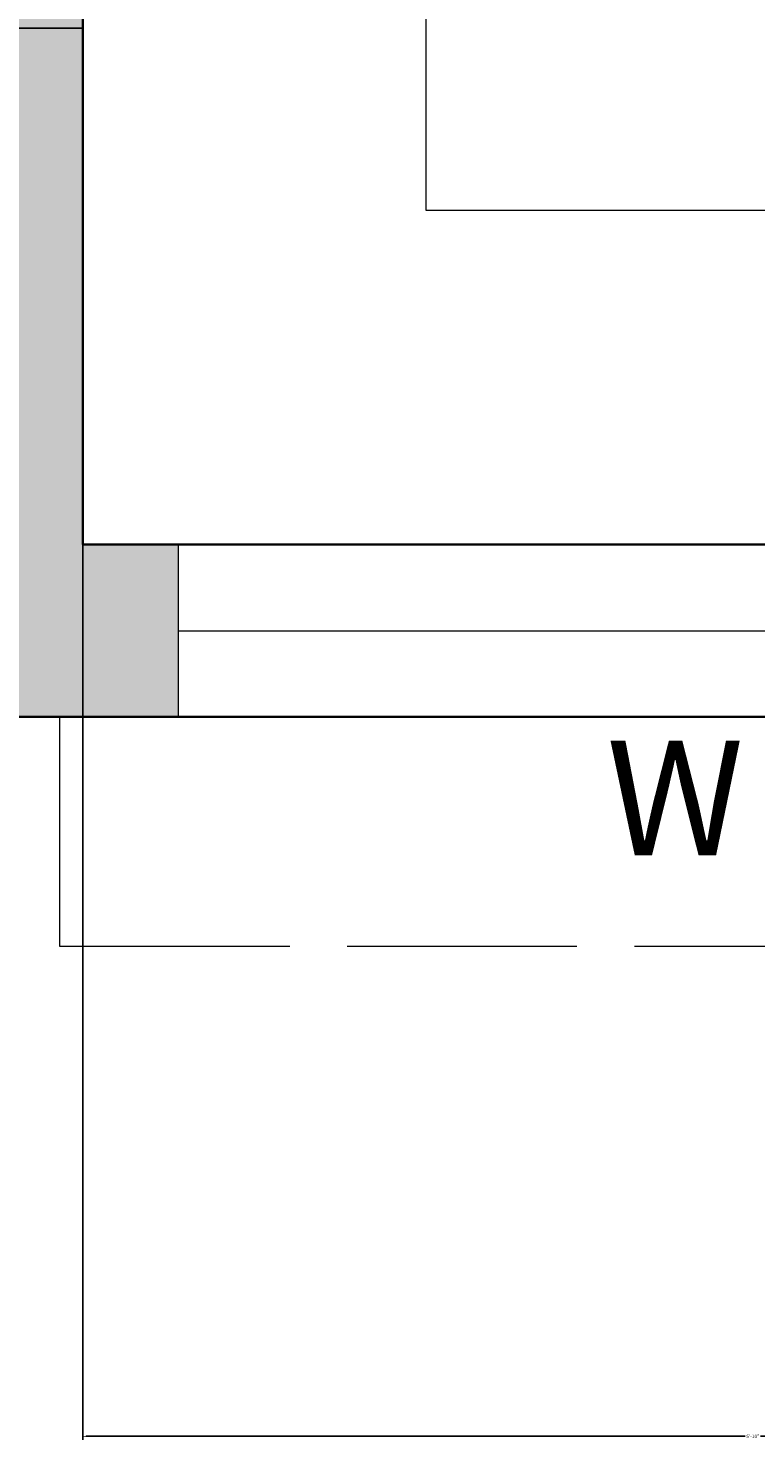
# Model space of a CAD drawing. Units: inches. Extents: x -5 to 482, y -460 to 66.
# Tile 10 of 31: x 142 to 180, y -460 to -386. Entities that reach past the tile are written whole.
import ezdxf

# ---------------------------------------------------------------- set-up
doc = ezdxf.new("R2010")
doc.units = ezdxf.units.IN
doc.header["$MEASUREMENT"] = 0
doc.linetypes.add('ACAD_ISO02W100', pattern=[15, 12, -3])
for name, color, linetype, lineweight in [('A-ANNO-DIMS', 2, 'Continuous', 18), ('A-ANNO-SYMB', 7, 'Continuous', 18), ('A-ANNO-TEXT', 7, 'Continuous', 18), ('A-GLAZ', 4, 'Continuous', 18), ('A-GLAZ-OVHD', 4, 'ACAD_ISO02W100', 13), ('A-WALL', 7, 'Continuous', 35), ('A-WALL-PATT', 152, 'Continuous', 13)]:
    doc.layers.add(name, color=color, linetype=linetype, lineweight=lineweight)
doc.styles.get("Standard").update_dxf_attribs({"font": 'arial.ttf'})
doc.dimstyles.get("Standard").update_dxf_attribs({"dimtxt": 0.18, "dimasz": 0.18, "dimexe": 0.18, "dimexo": 0.0625, "dimgap": 0.09, "dimtad": 0, "dimtih": 1, "dimtoh": 1, "dimdec": 0, "dimzin": 0, "dimdsep": 46, "dimlunit": 3, "dimtxsty": 'Standard', "dimcen": 0.09, "dimadec": 0, "dimazin": 0, "dimtfac": 1, "dimtdec": 0, "dimtofl": 0, "dimtmove": 0, "dimatfit": 3, "dimfxl": 1, "dimtolj": 1, "dimtzin": 0, "dimarcsym": 0})

# ---------------------------------------------------------------- blocks, each defined once
blk = doc.blocks.new('WIN-GLAZ-60IN')
for p, q in [((0, 9), (60, 9)), ((0, 4.5), (60, 4.5)), ((60, 0), (0, 0))]:
    blk.add_line(p, q)
blk = doc.blocks.new('WIN-SHADE-72IN')
for p, q in [((0, 12), (72, 12)), ((0, 12), (0, 0)), ((72, 12), (72, 0))]:
    blk.add_line(p, q)
blk = doc.blocks.new('*D71')
at = {"layer": 'A-ANNO-DIMS', "color": 0, "lineweight": -2, "transparency": 16777216}
for p, q in [((144.377, -385.924), (144.377, -459.629)), ((214.377, -385.924), (214.377, -459.629)), ((144.557, -459.449), (178.978, -459.449)), ((214.197, -459.449), (179.776, -459.449))]:
    blk.add_line(p, q, dxfattribs=at)
at = {"layer": 'A-ANNO-DIMS', "color": 0, "transparency": 16777216}
for points in [[(144.557, -459.419), (144.557, -459.479), (144.377, -459.449)], [(214.197, -459.419), (214.197, -459.479), (214.377, -459.449)]]:
    blk.add_solid(points, dxfattribs=at)
at = {"layer": 'Defpoints', "color": 0, "transparency": 16777216}
for p in [(144.377, -385.861), (214.377, -385.861), (214.377, -459.449)]:
    blk.add_point(p, dxfattribs=at)
at = {"layer": 'A-ANNO-DIMS', "color": 0, "transparency": 16777216, "insert": (179.377, -459.449), "char_height": 0.18, "attachment_point": 5}
blk.add_mtext('\\A1;5\'-10"', dxfattribs=at)
blk = doc.blocks.new('*D72')
at = {"layer": 'A-ANNO-DIMS', "color": 0, "lineweight": -2, "transparency": 16777216}
for p, q in [((144.314, -375.861), (-4.903, -375.861)), ((-4.723, -376.041), (-4.723, -380.679)), ((-4.723, -385.681), (-4.723, -381.043)), ((144.314, -385.861), (-4.903, -385.861))]:
    blk.add_line(p, q, dxfattribs=at)
at = {"layer": 'A-ANNO-DIMS', "color": 0, "transparency": 16777216}
for points in [[(-4.753, -376.041), (-4.693, -376.041), (-4.723, -375.861)], [(-4.753, -385.681), (-4.693, -385.681), (-4.723, -385.861)]]:
    blk.add_solid(points, dxfattribs=at)
at = {"layer": 'Defpoints', "color": 0, "transparency": 16777216}
for p in [(144.377, -375.861), (-4.723, -385.861), (144.377, -385.861)]:
    blk.add_point(p, dxfattribs=at)
at = {"layer": 'A-ANNO-DIMS', "color": 0, "transparency": 16777216, "insert": (-4.723, -380.861), "char_height": 0.18, "attachment_point": 5}
blk.add_mtext('\\A1;0\'-10"', dxfattribs=at)

msp = doc.modelspace()

# ---------------------------------------------------------------- hatches: boundary and pattern name
at = {"layer": 'A-WALL-PATT'}
h = msp.add_hatch(color=256, dxfattribs=at)
h.dxf.hatch_style = 1
h.paths.add_polyline_path([(149.377, -412.849), (144.377, -412.849), (144.377, -283.849), (144.377, -279.349), (133.877, -279.349), (133.877, -283.849), (139.877, -283.849), (139.877, -412.849), (133.51, -412.849), (133.51, -413.916), (102.652, -413.916), (102.652, -421.02), (133.51, -421.02), (133.51, -421.849), (149.377, -421.849)])
h.paths.add_polyline_path([(226.054, -412.849), (218.877, -412.849), (218.877, -350.849), (262.877, -350.849), (262.877, -386.849), (267.377, -386.849), (267.377, -283.849), (270.377, -283.849), (270.377, -279.349), (244.877, -279.349), (244.877, -283.849), (262.877, -283.849), (262.877, -346.349), (218.877, -346.349), (218.877, -283.849), (220.877, -283.849), (220.877, -279.349), (214.377, -279.349), (214.377, -283.849), (214.377, -412.849), (209.377, -412.849), (209.377, -421.849), (226.054, -421.849)])
h.paths.add_polyline_path([(315.815, -412.849), (250.054, -412.849), (250.054, -421.849), (315.815, -421.849)])
h.paths.add_polyline_path([(430.377, -378.349), (421.377, -378.349), (421.377, -412.849), (375.815, -412.849), (375.815, -421.849), (430.377, -421.849)])
h.paths.add_polyline_path([(78.691, -413.916), (47.68, -413.916), (47.68, -412.849), (41.877, -412.849), (41.877, -283.849), (109.877, -283.849), (109.877, -279.349), (41.877, -279.349), (41.877, -241.849), (32.877, -241.849), (32.877, -421.849), (47.68, -421.849), (47.68, -421.02), (78.691, -421.02)])
h.paths.add_polyline_path([(41.877, -144.349), (154.377, -144.349), (154.377, -137.849), (149.877, -137.849), (149.877, -139.849), (41.877, -139.849), (41.877, -97.849), (32.877, -97.849), (32.877, -181.849), (41.877, -181.849)])
h.paths.add_polyline_path([(430.377, -241.849), (421.377, -241.849), (421.377, -279.349), (309.377, -279.349), (309.377, -170.349), (304.877, -170.349), (304.877, -279.349), (294.377, -279.349), (294.377, -283.849), (421.377, -283.849), (421.377, -318.349), (430.377, -318.349)])
h.paths.add_polyline_path([(430.377, -119.849), (421.377, -119.849), (421.377, -139.849), (419.377, -139.849), (419.377, -144.349), (421.377, -144.349), (421.377, -181.849), (430.377, -181.849)])
h.paths.add_polyline_path([(395.377, -139.849), (377.377, -139.849), (377.377, -75.849), (421.377, -75.849), (421.377, -95.849), (430.377, -95.849), (430.377, -45.599), (421.377, -45.599), (421.377, -71.349), (377.377, -71.349), (377.377, -22.849), (372.877, -22.849), (372.877, -139.849), (242.877, -139.849), (242.877, -137.849), (238.377, -137.849), (238.377, -144.349), (304.877, -144.349), (304.877, -146.349), (309.377, -146.349), (309.377, -144.349), (395.377, -144.349)])
h.paths.add_polyline_path([(65.877, 13.151), (32.877, 13.151), (32.877, -37.849), (41.877, -37.849), (41.877, 4.151), (65.877, 4.151)])
h.paths.add_polyline_path([(166.377, 13.151), (125.877, 13.151), (125.877, 4.151), (149.877, 4.151), (149.877, -113.849), (154.377, -113.849), (154.377, 4.151), (166.377, 4.151)])
h.paths.add_polyline_path([(277.877, 13.151), (226.377, 13.151), (226.377, 4.151), (238.377, 4.151), (238.377, -113.849), (242.877, -113.849), (242.877, 4.151), (277.877, 4.151)])
h.paths.add_polyline_path([(430.377, 13.151), (337.877, 13.151), (337.877, 4.151), (372.877, 4.151), (372.877, 1.151), (377.377, 1.151), (377.377, 4.151), (421.377, 4.151), (421.377, -21.599), (430.377, -21.599)])

# ---------------------------------------------------------------- linework, layer by layer
at = {"layer": 'A-ANNO-SYMB'}
for p, q in [((162.322, -395.385), (162.322, -315.861)), ((197.881, -395.385), (162.322, -395.385))]:
    msp.add_line(p, q, dxfattribs=at)
at = {"layer": 'A-GLAZ'}
msp.add_line((149.377, -421.849), (149.377, -412.849), dxfattribs=at)
at = {"layer": 'A-WALL'}
for p, q in [((144.377, -283.849), (144.377, -412.849)), ((144.377, -412.849), (214.377, -412.849)), ((133.51, -421.849), (430.377, -421.849))]:
    msp.add_line(p, q, dxfattribs=at)

# ---------------------------------------------------------------- block references
at = {"layer": 'A-GLAZ'}
msp.add_blockref('WIN-GLAZ-60IN', (149.377, -421.849), dxfattribs=at)
at = {"layer": 'A-GLAZ-OVHD', "rotation": 180}
msp.add_blockref('WIN-SHADE-72IN', (215.191, -421.848), dxfattribs=at)

# ---------------------------------------------------------------- texts
at = {"layer": 'A-ANNO-TEXT', "insert": (171.729, -423.085), "char_height": 6, "attachment_point": 1}
msp.add_mtext('W', dxfattribs=at)

# ---------------------------------------------------------------- dimensions: what is measured, and where the dimension line sits
at = {"layer": 'A-ANNO-DIMS'}
dim = msp.add_linear_dim(base=(-4.723, -385.861), p1=(144.377, -375.861), p2=(144.377, -385.861), angle=90, dimstyle='Standard', override={"dimdec": 1, "dimlfac": 1, "dimrnd": 0, "dimzin": 1, "dimdsep": 46, "dimlunit": 4, "dimfrac": 2}, dxfattribs=at)
dim.commit()
dim.dimension.update_dxf_attribs({"geometry": '*D72', "text_midpoint": (-4.723, -380.861)})
dim = msp.add_linear_dim(base=(214.377, -459.449), p1=(144.377, -385.861), p2=(214.377, -385.861), dimstyle='Standard', override={"dimdec": 1, "dimlfac": 1, "dimrnd": 0, "dimzin": 1, "dimdsep": 46, "dimlunit": 4, "dimfrac": 2}, dxfattribs=at)
dim.commit()
dim.dimension.update_dxf_attribs({"geometry": '*D71', "text_midpoint": (179.377, -459.449)})

doc.saveas('drawing.dxf')
